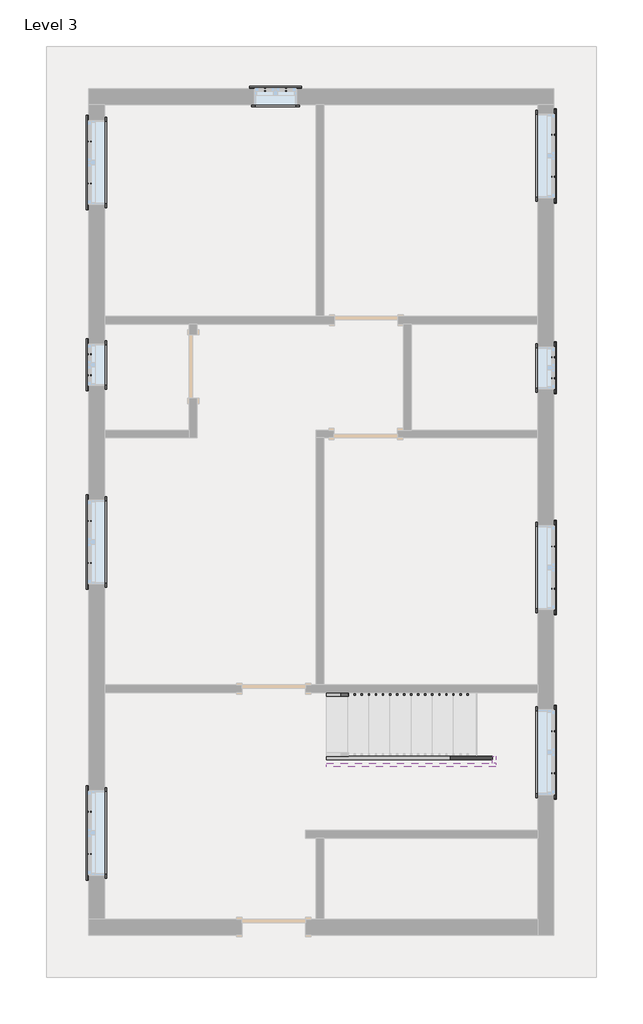
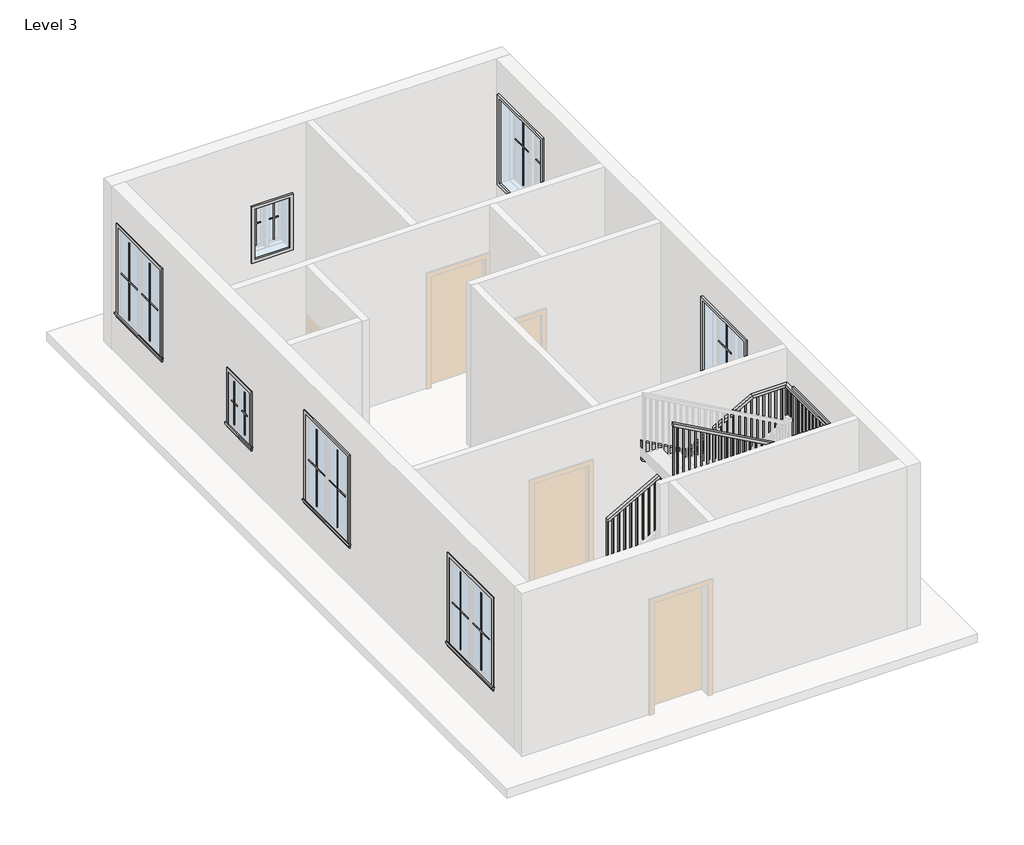
# One storey, part 2 of 2: 36 proxies, 3 members, 1 railing.
"""IFC4 building model written with IfcOpenShell, lengths in millimetres."""

from ifc_helpers import new_model, si_unit, frame, origin, place, context, project, spatial, polyline, outline, extrude, faceted_brep, transform, mapped, element, save
from components import muntin_pattern_2x2_muntin_pattern_2x2_6dad3731, muntin_pattern_2x2_muntin_pattern_2x2_a30a3345, muntin_pattern_2x2_muntin_pattern_2x2_53152e2c, muntin_pattern_2x2_muntin_pattern_2x2_e8f3e573, trim_window_exterior_flat_with_sill_92b9b949, trim_window_exterior_flat_with_sill_a665a915, trim_window_interior_flat_picture_frame_3bb882cf, trim_window_interior_flat_picture_frame_d485c387

model = new_model("IFC4")

# Units and contexts
model_context = context("Model", 3, world=origin())
ifc_project = project(units=[si_unit("LENGTHUNIT", "METRE", prefix="MILLI")], contexts=[model_context])

# Site, building, storey
site = spatial("IfcSite", under=ifc_project)
building = spatial("IfcBuilding", under=site)
storey = spatial("IfcBuildingStorey", under=building, Name="Level 3", Elevation=6096.0)

# Proxies
placement = place(None, origin())
muntin_pattern_2x2_muntin_pattern_2x2_shape = muntin_pattern_2x2_muntin_pattern_2x2_6dad3731(model_context)
element("IfcBuildingElementProxy", 1, Name="Muntin Pattern_2x2 : Muntin Pattern_2x2", ObjectType="Muntin Pattern_2x2 : Muntin Pattern_2x2", at=placement, inside=storey, context=model_context, shape_type="MappedRepresentation", body=[
    mapped(muntin_pattern_2x2_muntin_pattern_2x2_shape, transform((1279.525, 2947.4914062, 7080.25), x_axis=(0.0, 1.0, 0.0), y_axis=(-1.0, 0.0, 0.0), z_axis=(0.0, 0.0, 1.0))),
])
element("IfcBuildingElementProxy", 2, Name="Muntin Pattern_2x2 : Muntin Pattern_2x2", ObjectType="Muntin Pattern_2x2 : Muntin Pattern_2x2", at=placement, inside=storey, context=model_context, shape_type="MappedRepresentation", body=[
    mapped(muntin_pattern_2x2_muntin_pattern_2x2_shape, transform((1279.525, 7138.4914062, 7080.25), x_axis=(0.0, 1.0, 0.0), y_axis=(-1.0, 0.0, 0.0), z_axis=(0.0, 0.0, 1.0))),
])
element("IfcBuildingElementProxy", 3, Name="Muntin Pattern_2x2 : Muntin Pattern_2x2", ObjectType="Muntin Pattern_2x2 : Muntin Pattern_2x2", at=placement, inside=storey, context=model_context, shape_type="MappedRepresentation", body=[
    mapped(muntin_pattern_2x2_muntin_pattern_2x2_shape, transform((1279.525, 12605.8414062, 7080.25), x_axis=(0.0, 1.0, 0.0), y_axis=(-1.0, 0.0, 0.0), z_axis=(0.0, 0.0, 1.0))),
])
element("IfcBuildingElementProxy", 4, Name="Muntin Pattern_2x2 : Muntin Pattern_2x2", ObjectType="Muntin Pattern_2x2 : Muntin Pattern_2x2", at=placement, inside=storey, context=model_context, shape_type="MappedRepresentation", body=[
    mapped(muntin_pattern_2x2_muntin_pattern_2x2_shape, transform((7966.075, 13308.0125, 7080.25), x_axis=(0.0, -1.0, 0.0), y_axis=(1.0, 0.0, 0.0), z_axis=(0.0, 0.0, 1.0))),
])
element("IfcBuildingElementProxy", 5, Name="Muntin Pattern_2x2 : Muntin Pattern_2x2", ObjectType="Muntin Pattern_2x2 : Muntin Pattern_2x2", at=placement, inside=storey, context=model_context, shape_type="MappedRepresentation", body=[
    mapped(muntin_pattern_2x2_muntin_pattern_2x2_shape, transform((7966.075, 7377.1125, 7080.25), x_axis=(0.0, -1.0, 0.0), y_axis=(1.0, 0.0, 0.0), z_axis=(0.0, 0.0, 1.0))),
])
element("IfcBuildingElementProxy", 6, Name="Muntin Pattern_2x2 : Muntin Pattern_2x2", ObjectType="Muntin Pattern_2x2 : Muntin Pattern_2x2", at=placement, inside=storey, context=model_context, shape_type="MappedRepresentation", body=[
    mapped(muntin_pattern_2x2_muntin_pattern_2x2_shape, transform((7966.075, 4716.4625, 7080.25), x_axis=(0.0, -1.0, 0.0), y_axis=(1.0, 0.0, 0.0), z_axis=(0.0, 0.0, 1.0))),
])
muntin_pattern_2x2_muntin_pattern_2x2_2_shape = muntin_pattern_2x2_muntin_pattern_2x2_a30a3345(model_context)
element("IfcBuildingElementProxy", 7, Name="Muntin Pattern_2x2 : Muntin Pattern_2x2", ObjectType="Muntin Pattern_2x2 : Muntin Pattern_2x2", at=placement, inside=storey, context=model_context, shape_type="MappedRepresentation", body=[
    mapped(muntin_pattern_2x2_muntin_pattern_2x2_2_shape, transform((1279.525, 3553.9164063, 7080.25), x_axis=(0.0, -1.0, 0.0), y_axis=(1.0, 0.0, 0.0), z_axis=(0.0, 0.0, 1.0))),
])
element("IfcBuildingElementProxy", 8, Name="Muntin Pattern_2x2 : Muntin Pattern_2x2", ObjectType="Muntin Pattern_2x2 : Muntin Pattern_2x2", at=placement, inside=storey, context=model_context, shape_type="MappedRepresentation", body=[
    mapped(muntin_pattern_2x2_muntin_pattern_2x2_2_shape, transform((1279.525, 7744.9164062, 7080.25), x_axis=(0.0, -1.0, 0.0), y_axis=(1.0, 0.0, 0.0), z_axis=(0.0, 0.0, 1.0))),
])
element("IfcBuildingElementProxy", 9, Name="Muntin Pattern_2x2 : Muntin Pattern_2x2", ObjectType="Muntin Pattern_2x2 : Muntin Pattern_2x2", at=placement, inside=storey, context=model_context, shape_type="MappedRepresentation", body=[
    mapped(muntin_pattern_2x2_muntin_pattern_2x2_2_shape, transform((1279.525, 13212.2664062, 7080.25), x_axis=(0.0, -1.0, 0.0), y_axis=(1.0, 0.0, 0.0), z_axis=(0.0, 0.0, 1.0))),
])
element("IfcBuildingElementProxy", 10, Name="Muntin Pattern_2x2 : Muntin Pattern_2x2", ObjectType="Muntin Pattern_2x2 : Muntin Pattern_2x2", at=placement, inside=storey, context=model_context, shape_type="MappedRepresentation", body=[
    mapped(muntin_pattern_2x2_muntin_pattern_2x2_2_shape, transform((7966.075, 12701.5875, 7080.25), x_axis=(0.0, 1.0, 0.0), y_axis=(-1.0, 0.0, 0.0), z_axis=(0.0, 0.0, 1.0))),
])
element("IfcBuildingElementProxy", 11, Name="Muntin Pattern_2x2 : Muntin Pattern_2x2", ObjectType="Muntin Pattern_2x2 : Muntin Pattern_2x2", at=placement, inside=storey, context=model_context, shape_type="MappedRepresentation", body=[
    mapped(muntin_pattern_2x2_muntin_pattern_2x2_2_shape, transform((7966.075, 6770.6875, 7080.25), x_axis=(0.0, 1.0, 0.0), y_axis=(-1.0, 0.0, 0.0), z_axis=(0.0, 0.0, 1.0))),
])
element("IfcBuildingElementProxy", 12, Name="Muntin Pattern_2x2 : Muntin Pattern_2x2", ObjectType="Muntin Pattern_2x2 : Muntin Pattern_2x2", at=placement, inside=storey, context=model_context, shape_type="MappedRepresentation", body=[
    mapped(muntin_pattern_2x2_muntin_pattern_2x2_2_shape, transform((7966.075, 4110.0375, 7080.25), x_axis=(0.0, 1.0, 0.0), y_axis=(-1.0, 0.0, 0.0), z_axis=(0.0, 0.0, 1.0))),
])
muntin_pattern_2x2_muntin_pattern_2x2_3_shape = muntin_pattern_2x2_muntin_pattern_2x2_53152e2c(model_context)
element("IfcBuildingElementProxy", 13, Name="Muntin Pattern_2x2 : Muntin Pattern_2x2", ObjectType="Muntin Pattern_2x2 : Muntin Pattern_2x2", at=placement, inside=storey, context=model_context, shape_type="MappedRepresentation", body=[
    mapped(muntin_pattern_2x2_muntin_pattern_2x2_3_shape, transform((3811.5875, 13960.475, 7080.25), x_axis=(1.0, 0.0, 0.0), y_axis=(0.0, 1.0, 0.0), z_axis=(0.0, 0.0, 1.0))),
])
element("IfcBuildingElementProxy", 14, Name="Muntin Pattern_2x2 : Muntin Pattern_2x2", ObjectType="Muntin Pattern_2x2 : Muntin Pattern_2x2", at=placement, inside=storey, context=model_context, shape_type="MappedRepresentation", body=[
    mapped(muntin_pattern_2x2_muntin_pattern_2x2_3_shape, transform((7966.075, 10101.2625, 7080.25), x_axis=(0.0, -1.0, 0.0), y_axis=(1.0, 0.0, 0.0), z_axis=(0.0, 0.0, 1.0))),
])
element("IfcBuildingElementProxy", 15, Name="Muntin Pattern_2x2 : Muntin Pattern_2x2", ObjectType="Muntin Pattern_2x2 : Muntin Pattern_2x2", at=placement, inside=storey, context=model_context, shape_type="MappedRepresentation", body=[
    mapped(muntin_pattern_2x2_muntin_pattern_2x2_3_shape, transform((1279.525, 9843.5914062, 7080.25), x_axis=(0.0, 1.0, 0.0), y_axis=(-1.0, 0.0, 0.0), z_axis=(0.0, 0.0, 1.0))),
])
muntin_pattern_2x2_muntin_pattern_2x2_4_shape = muntin_pattern_2x2_muntin_pattern_2x2_e8f3e573(model_context)
element("IfcBuildingElementProxy", 16, Name="Muntin Pattern_2x2 : Muntin Pattern_2x2", ObjectType="Muntin Pattern_2x2 : Muntin Pattern_2x2", at=placement, inside=storey, context=model_context, shape_type="MappedRepresentation", body=[
    mapped(muntin_pattern_2x2_muntin_pattern_2x2_4_shape, transform((4113.2125, 13960.475, 7080.25), x_axis=(-1.0, 0.0, 0.0), y_axis=(0.0, -1.0, 0.0), z_axis=(0.0, 0.0, 1.0))),
])
element("IfcBuildingElementProxy", 17, Name="Muntin Pattern_2x2 : Muntin Pattern_2x2", ObjectType="Muntin Pattern_2x2 : Muntin Pattern_2x2", at=placement, inside=storey, context=model_context, shape_type="MappedRepresentation", body=[
    mapped(muntin_pattern_2x2_muntin_pattern_2x2_4_shape, transform((7966.075, 9799.6375, 7080.25), x_axis=(0.0, 1.0, 0.0), y_axis=(-1.0, 0.0, 0.0), z_axis=(0.0, 0.0, 1.0))),
])
element("IfcBuildingElementProxy", 18, Name="Muntin Pattern_2x2 : Muntin Pattern_2x2", ObjectType="Muntin Pattern_2x2 : Muntin Pattern_2x2", at=placement, inside=storey, context=model_context, shape_type="MappedRepresentation", body=[
    mapped(muntin_pattern_2x2_muntin_pattern_2x2_4_shape, transform((1279.525, 10145.2164062, 7080.25), x_axis=(0.0, -1.0, 0.0), y_axis=(1.0, 0.0, 0.0), z_axis=(0.0, 0.0, 1.0))),
])
trim_window_exterior_flat_with_sill_shape = trim_window_exterior_flat_with_sill_92b9b949(model_context)
element("IfcBuildingElementProxy", 19, Name="Trim-Window-Exterior-Flat : with Sill", ObjectType="Trim-Window-Exterior-Flat : with Sill", at=placement, inside=storey, context=model_context, shape_type="MappedRepresentation", body=[
    mapped(trim_window_exterior_flat_with_sill_shape, transform((1270.0, 3250.7039063, 8534.4), x_axis=(0.0, -1.0, 0.0), y_axis=(0.0, 0.0, 1.0), z_axis=(-1.0, 0.0, 0.0))),
])
element("IfcBuildingElementProxy", 20, Name="Trim-Window-Exterior-Flat : with Sill", ObjectType="Trim-Window-Exterior-Flat : with Sill", at=placement, inside=storey, context=model_context, shape_type="MappedRepresentation", body=[
    mapped(trim_window_exterior_flat_with_sill_shape, transform((1270.0, 7441.7039063, 8534.4), x_axis=(0.0, -1.0, 0.0), y_axis=(0.0, 0.0, 1.0), z_axis=(-1.0, 0.0, 0.0))),
])
element("IfcBuildingElementProxy", 21, Name="Trim-Window-Exterior-Flat : with Sill", ObjectType="Trim-Window-Exterior-Flat : with Sill", at=placement, inside=storey, context=model_context, shape_type="MappedRepresentation", body=[
    mapped(trim_window_exterior_flat_with_sill_shape, transform((1270.0, 12909.0539063, 8534.4), x_axis=(0.0, -1.0, 0.0), y_axis=(0.0, 0.0, 1.0), z_axis=(-1.0, 0.0, 0.0))),
])
element("IfcBuildingElementProxy", 22, Name="Trim-Window-Exterior-Flat : with Sill", ObjectType="Trim-Window-Exterior-Flat : with Sill", at=placement, inside=storey, context=model_context, shape_type="MappedRepresentation", body=[
    mapped(trim_window_exterior_flat_with_sill_shape, transform((7975.6, 13004.8, 8534.4), x_axis=(0.0, 1.0, 0.0), y_axis=(0.0, 0.0, 1.0), z_axis=(1.0, 0.0, 0.0))),
])
element("IfcBuildingElementProxy", 23, Name="Trim-Window-Exterior-Flat : with Sill", ObjectType="Trim-Window-Exterior-Flat : with Sill", at=placement, inside=storey, context=model_context, shape_type="MappedRepresentation", body=[
    mapped(trim_window_exterior_flat_with_sill_shape, transform((7975.6, 7073.9, 8534.4), x_axis=(0.0, 1.0, 0.0), y_axis=(0.0, 0.0, 1.0), z_axis=(1.0, 0.0, 0.0))),
])
element("IfcBuildingElementProxy", 24, Name="Trim-Window-Exterior-Flat : with Sill", ObjectType="Trim-Window-Exterior-Flat : with Sill", at=placement, inside=storey, context=model_context, shape_type="MappedRepresentation", body=[
    mapped(trim_window_exterior_flat_with_sill_shape, transform((7975.6, 4413.25, 8534.4), x_axis=(0.0, 1.0, 0.0), y_axis=(0.0, 0.0, 1.0), z_axis=(1.0, 0.0, 0.0))),
])
trim_window_exterior_flat_with_sill_2_shape = trim_window_exterior_flat_with_sill_a665a915(model_context)
element("IfcBuildingElementProxy", 25, Name="Trim-Window-Exterior-Flat : with Sill", ObjectType="Trim-Window-Exterior-Flat : with Sill", at=placement, inside=storey, context=model_context, shape_type="MappedRepresentation", body=[
    mapped(trim_window_exterior_flat_with_sill_2_shape, transform((3962.4, 13970.0, 7924.8), x_axis=(-1.0, 0.0, 0.0), y_axis=(0.0, 0.0, 1.0), z_axis=(0.0, 1.0, 0.0))),
])
element("IfcBuildingElementProxy", 26, Name="Trim-Window-Exterior-Flat : with Sill", ObjectType="Trim-Window-Exterior-Flat : with Sill", at=placement, inside=storey, context=model_context, shape_type="MappedRepresentation", body=[
    mapped(trim_window_exterior_flat_with_sill_2_shape, transform((7975.6, 9950.45, 7924.8), x_axis=(0.0, 1.0, 0.0), y_axis=(0.0, 0.0, 1.0), z_axis=(1.0, 0.0, 0.0))),
])
element("IfcBuildingElementProxy", 27, Name="Trim-Window-Exterior-Flat : with Sill", ObjectType="Trim-Window-Exterior-Flat : with Sill", at=placement, inside=storey, context=model_context, shape_type="MappedRepresentation", body=[
    mapped(trim_window_exterior_flat_with_sill_2_shape, transform((1270.0, 9994.4039062, 7924.8), x_axis=(0.0, -1.0, 0.0), y_axis=(0.0, 0.0, 1.0), z_axis=(-1.0, 0.0, 0.0))),
])
trim_window_interior_flat_picture_frame_shape = trim_window_interior_flat_picture_frame_3bb882cf(model_context)
element("IfcBuildingElementProxy", 28, Name="Trim-Window-Interior-Flat : Picture Frame", ObjectType="Trim-Window-Interior-Flat : Picture Frame", at=placement, inside=storey, context=model_context, shape_type="MappedRepresentation", body=[
    mapped(trim_window_interior_flat_picture_frame_shape, transform((1498.6, 3250.7039063, 8534.4), x_axis=(0.0, 1.0, 0.0), y_axis=(0.0, 0.0, 1.0), z_axis=(1.0, 0.0, 0.0))),
])
element("IfcBuildingElementProxy", 29, Name="Trim-Window-Interior-Flat : Picture Frame", ObjectType="Trim-Window-Interior-Flat : Picture Frame", at=placement, inside=storey, context=model_context, shape_type="MappedRepresentation", body=[
    mapped(trim_window_interior_flat_picture_frame_shape, transform((1498.6, 7441.7039062, 8534.4), x_axis=(0.0, 1.0, 0.0), y_axis=(0.0, 0.0, 1.0), z_axis=(1.0, 0.0, 0.0))),
])
element("IfcBuildingElementProxy", 30, Name="Trim-Window-Interior-Flat : Picture Frame", ObjectType="Trim-Window-Interior-Flat : Picture Frame", at=placement, inside=storey, context=model_context, shape_type="MappedRepresentation", body=[
    mapped(trim_window_interior_flat_picture_frame_shape, transform((1498.6, 12909.0539062, 8534.4), x_axis=(0.0, 1.0, 0.0), y_axis=(0.0, 0.0, 1.0), z_axis=(1.0, 0.0, 0.0))),
])
element("IfcBuildingElementProxy", 31, Name="Trim-Window-Interior-Flat : Picture Frame", ObjectType="Trim-Window-Interior-Flat : Picture Frame", at=placement, inside=storey, context=model_context, shape_type="MappedRepresentation", body=[
    mapped(trim_window_interior_flat_picture_frame_shape, transform((7747.0, 13004.8, 8534.4), x_axis=(0.0, -1.0, 0.0), y_axis=(0.0, 0.0, 1.0), z_axis=(-1.0, 0.0, 0.0))),
])
element("IfcBuildingElementProxy", 32, Name="Trim-Window-Interior-Flat : Picture Frame", ObjectType="Trim-Window-Interior-Flat : Picture Frame", at=placement, inside=storey, context=model_context, shape_type="MappedRepresentation", body=[
    mapped(trim_window_interior_flat_picture_frame_shape, transform((7747.0, 7073.9, 8534.4), x_axis=(0.0, -1.0, 0.0), y_axis=(0.0, 0.0, 1.0), z_axis=(-1.0, 0.0, 0.0))),
])
element("IfcBuildingElementProxy", 33, Name="Trim-Window-Interior-Flat : Picture Frame", ObjectType="Trim-Window-Interior-Flat : Picture Frame", at=placement, inside=storey, context=model_context, shape_type="MappedRepresentation", body=[
    mapped(trim_window_interior_flat_picture_frame_shape, transform((7747.0, 4413.25, 8534.4), x_axis=(0.0, -1.0, 0.0), y_axis=(0.0, 0.0, 1.0), z_axis=(-1.0, 0.0, 0.0))),
])
trim_window_interior_flat_picture_frame_2_shape = trim_window_interior_flat_picture_frame_d485c387(model_context)
element("IfcBuildingElementProxy", 34, Name="Trim-Window-Interior-Flat : Picture Frame", ObjectType="Trim-Window-Interior-Flat : Picture Frame", at=placement, inside=storey, context=model_context, shape_type="MappedRepresentation", body=[
    mapped(trim_window_interior_flat_picture_frame_2_shape, transform((3962.4, 13741.4, 7924.8), x_axis=(1.0, 0.0, 0.0), y_axis=(0.0, 0.0, 1.0), z_axis=(0.0, -1.0, 0.0))),
])
element("IfcBuildingElementProxy", 35, Name="Trim-Window-Interior-Flat : Picture Frame", ObjectType="Trim-Window-Interior-Flat : Picture Frame", at=placement, inside=storey, context=model_context, shape_type="MappedRepresentation", body=[
    mapped(trim_window_interior_flat_picture_frame_2_shape, transform((7747.0, 9950.45, 7924.8), x_axis=(0.0, -1.0, 0.0), y_axis=(0.0, 0.0, 1.0), z_axis=(-1.0, 0.0, 0.0))),
])
element("IfcBuildingElementProxy", 36, Name="Trim-Window-Interior-Flat : Picture Frame", ObjectType="Trim-Window-Interior-Flat : Picture Frame", at=placement, inside=storey, context=model_context, shape_type="MappedRepresentation", body=[
    mapped(trim_window_interior_flat_picture_frame_2_shape, transform((1498.6, 9994.4039062, 7924.8), x_axis=(0.0, 1.0, 0.0), y_axis=(0.0, 0.0, 1.0), z_axis=(1.0, 0.0, 0.0))),
])

# Members
element("IfcMember", 37, ObjectType="Stringer - 2\" Width", at=placement, inside=storey, context=model_context, shape_type="SweptSolid", body=[
    extrude(outline(polyline([(6303.5983948, 4699.0), (6096.0, 4699.0), (6096.0, 4952.9445028), (7281.3641651, 7086.6), (7630.0428392, 7086.6), (6303.5983948, 4699.0)])), frame((0.0, 4305.3, 0.0), z_axis=(0.0, 1.0, 0.0), x_axis=(0.0, 0.0, 1.0)), (0.0, 0.0, 1.0), 50.8),
])
element("IfcMember", 38, ObjectType="Stringer - 2\" Width", at=placement, inside=storey, context=model_context, shape_type="SweptSolid", body=[
    extrude(outline(polyline([(7086.6, 4356.1), (7137.4, 4356.1), (7137.4, 4254.5), (7086.6, 4254.5), (7086.6, 4356.1)])), frame((0.0, 0.0, 7391.4), z_axis=(0.0, 0.0, 1.0), x_axis=(1.0, 0.0, 0.0)), (0.0, 0.0, 1.0), 304.8),
])
element("IfcMember", 39, ObjectType="Stringer - 2\" Width", at=placement, inside=storey, context=model_context, shape_type="SweptSolid", body=[
    extrude(outline(polyline([(7478.9197207, 7137.4), (7827.5983948, 7137.4), (9182.2650614, 4699.0), (8833.5863873, 4699.0), (7478.9197207, 7137.4)])), frame((0.0, 4203.7, 0.0), z_axis=(0.0, 1.0, 0.0), x_axis=(0.0, 0.0, 1.0)), (0.0, 0.0, 1.0), 50.8),
])

# Railing
element("IfcRailing", 40, ObjectType="Handrail - Rectangular", at=placement, inside=storey, context=model_context, shape_type="SolidModel", body=[
    faceted_brep([(4699.0, 5270.5, 7179.7333333), (4699.0, 5270.5, 7121.620221), (4699.0, 5219.7, 7121.620221), (4699.0, 5219.7, 7179.7333333), (7137.4, 5270.5, 8534.4), (7150.5636022, 5270.5, 8483.6), (7150.5636022, 5219.7, 8483.6), (7137.4, 5219.7, 8534.4), (7747.0, 5270.5, 8534.4), (7747.0, 5270.5, 8483.6), (7696.2, 5219.7, 8483.6), (7696.2, 5219.7, 8534.4), (7747.0, 3289.3, 8534.4), (7747.0, 3289.3, 8483.6), (7696.2, 3340.1, 8483.6), (7696.2, 3340.1, 8534.4), (7442.2, 3289.3, 8534.4), (7429.0363978, 3289.3, 8483.6), (7429.0363978, 3340.1, 8483.6), (7442.2, 3340.1, 8534.4), (4699.0, 3289.3, 10058.4), (4699.0, 3340.1, 10058.4), (4699.0, 3340.1, 10000.2868876), (4699.0, 3289.3, 10000.2868876)], [[[0, 1, 2, 3]], [[1, 0, 4, 5]], [[2, 1, 5, 6]], [[3, 2, 6, 7]], [[0, 3, 7, 4]], [[5, 4, 8, 9]], [[6, 5, 9, 10]], [[7, 6, 10, 11]], [[4, 7, 11, 8]], [[9, 8, 12, 13]], [[10, 9, 13, 14]], [[11, 10, 14, 15]], [[8, 11, 15, 12]], [[13, 12, 16, 17]], [[14, 13, 17, 18]], [[15, 14, 18, 19]], [[12, 15, 19, 16]], [[20, 21, 22, 23]], [[17, 16, 20, 23]], [[18, 17, 23, 22]], [[19, 18, 22, 21]], [[16, 19, 21, 20]]]),
    extrude(outline(polyline([(9963.245221, 4765.675), (8974.6666667, 4765.675), (8974.6666667, 4784.725), (9952.6618876, 4784.725), (9963.245221, 4765.675)])), frame((0.0, 3305.175, 0.0), z_axis=(0.0, 1.0, 0.0), x_axis=(0.0, 0.0, 1.0)), (0.0, 0.0, 1.0), 19.05),
    extrude(outline(polyline([(9906.8007765, 4867.275), (8974.6666667, 4867.275), (8974.6666667, 4886.325), (9896.2174432, 4886.325), (9906.8007765, 4867.275)])), frame((0.0, 3305.175, 0.0), z_axis=(0.0, 1.0, 0.0), x_axis=(0.0, 0.0, 1.0)), (0.0, 0.0, 1.0), 19.05),
    extrude(outline(polyline([(9850.3563321, 4968.875), (8974.6666667, 4968.875), (8974.6666667, 4987.925), (9839.7729988, 4987.925), (9850.3563321, 4968.875)])), frame((0.0, 3305.175, 0.0), z_axis=(0.0, 1.0, 0.0), x_axis=(0.0, 0.0, 1.0)), (0.0, 0.0, 1.0), 19.05),
    extrude(outline(polyline([(9793.9118876, 5070.475), (8805.3333333, 5070.475), (8805.3333333, 5089.525), (9783.3285543, 5089.525), (9793.9118876, 5070.475)])), frame((0.0, 3305.175, 0.0), z_axis=(0.0, 1.0, 0.0), x_axis=(0.0, 0.0, 1.0)), (0.0, 0.0, 1.0), 19.05),
    extrude(outline(polyline([(9737.4674432, 5172.075), (8805.3333333, 5172.075), (8805.3333333, 5191.125), (9726.8841099, 5191.125), (9737.4674432, 5172.075)])), frame((0.0, 3305.175, 0.0), z_axis=(0.0, 1.0, 0.0), x_axis=(0.0, 0.0, 1.0)), (0.0, 0.0, 1.0), 19.05),
    extrude(outline(polyline([(9681.0229988, 5273.675), (8805.3333333, 5273.675), (8805.3333333, 5292.725), (9670.4396654, 5292.725), (9681.0229988, 5273.675)])), frame((0.0, 3305.175, 0.0), z_axis=(0.0, 1.0, 0.0), x_axis=(0.0, 0.0, 1.0)), (0.0, 0.0, 1.0), 19.05),
    extrude(outline(polyline([(9624.5785543, 5375.275), (8636.0, 5375.275), (8636.0, 5394.325), (9613.995221, 5394.325), (9624.5785543, 5375.275)])), frame((0.0, 3305.175, 0.0), z_axis=(0.0, 1.0, 0.0), x_axis=(0.0, 0.0, 1.0)), (0.0, 0.0, 1.0), 19.05),
    extrude(outline(polyline([(9568.1341099, 5476.875), (8636.0, 5476.875), (8636.0, 5495.925), (9557.5507765, 5495.925), (9568.1341099, 5476.875)])), frame((0.0, 3305.175, 0.0), z_axis=(0.0, 1.0, 0.0), x_axis=(0.0, 0.0, 1.0)), (0.0, 0.0, 1.0), 19.05),
    extrude(outline(polyline([(9511.6896654, 5578.475), (8636.0, 5578.475), (8636.0, 5597.525), (9501.1063321, 5597.525), (9511.6896654, 5578.475)])), frame((0.0, 3305.175, 0.0), z_axis=(0.0, 1.0, 0.0), x_axis=(0.0, 0.0, 1.0)), (0.0, 0.0, 1.0), 19.05),
    extrude(outline(polyline([(9455.245221, 5680.075), (8466.6666667, 5680.075), (8466.6666667, 5699.125), (9444.6618876, 5699.125), (9455.245221, 5680.075)])), frame((0.0, 3305.175, 0.0), z_axis=(0.0, 1.0, 0.0), x_axis=(0.0, 0.0, 1.0)), (0.0, 0.0, 1.0), 19.05),
    extrude(outline(polyline([(9398.8007765, 5781.675), (8466.6666667, 5781.675), (8466.6666667, 5800.725), (9388.2174432, 5800.725), (9398.8007765, 5781.675)])), frame((0.0, 3305.175, 0.0), z_axis=(0.0, 1.0, 0.0), x_axis=(0.0, 0.0, 1.0)), (0.0, 0.0, 1.0), 19.05),
    extrude(outline(polyline([(9342.3563321, 5883.275), (8466.6666667, 5883.275), (8466.6666667, 5902.325), (9331.7729988, 5902.325), (9342.3563321, 5883.275)])), frame((0.0, 3305.175, 0.0), z_axis=(0.0, 1.0, 0.0), x_axis=(0.0, 0.0, 1.0)), (0.0, 0.0, 1.0), 19.05),
    extrude(outline(polyline([(9285.9118876, 5984.875), (8297.3333333, 5984.875), (8297.3333333, 6003.925), (9275.3285543, 6003.925), (9285.9118876, 5984.875)])), frame((0.0, 3305.175, 0.0), z_axis=(0.0, 1.0, 0.0), x_axis=(0.0, 0.0, 1.0)), (0.0, 0.0, 1.0), 19.05),
    extrude(outline(polyline([(9229.4674432, 6086.475), (8297.3333333, 6086.475), (8297.3333333, 6105.525), (9218.8841099, 6105.525), (9229.4674432, 6086.475)])), frame((0.0, 3305.175, 0.0), z_axis=(0.0, 1.0, 0.0), x_axis=(0.0, 0.0, 1.0)), (0.0, 0.0, 1.0), 19.05),
    extrude(outline(polyline([(9173.0229988, 6188.075), (8297.3333333, 6188.075), (8297.3333333, 6207.125), (9162.4396654, 6207.125), (9173.0229988, 6188.075)])), frame((0.0, 3305.175, 0.0), z_axis=(0.0, 1.0, 0.0), x_axis=(0.0, 0.0, 1.0)), (0.0, 0.0, 1.0), 19.05),
    extrude(outline(polyline([(9116.5785543, 6289.675), (8128.0, 6289.675), (8128.0, 6308.725), (9105.995221, 6308.725), (9116.5785543, 6289.675)])), frame((0.0, 3305.175, 0.0), z_axis=(0.0, 1.0, 0.0), x_axis=(0.0, 0.0, 1.0)), (0.0, 0.0, 1.0), 19.05),
    extrude(outline(polyline([(9060.1341099, 6391.275), (8128.0, 6391.275), (8128.0, 6410.325), (9049.5507765, 6410.325), (9060.1341099, 6391.275)])), frame((0.0, 3305.175, 0.0), z_axis=(0.0, 1.0, 0.0), x_axis=(0.0, 0.0, 1.0)), (0.0, 0.0, 1.0), 19.05),
    extrude(outline(polyline([(9003.6896654, 6492.875), (8128.0, 6492.875), (8128.0, 6511.925), (8993.1063321, 6511.925), (9003.6896654, 6492.875)])), frame((0.0, 3305.175, 0.0), z_axis=(0.0, 1.0, 0.0), x_axis=(0.0, 0.0, 1.0)), (0.0, 0.0, 1.0), 19.05),
    extrude(outline(polyline([(8947.245221, 6594.475), (7958.6666667, 6594.475), (7958.6666667, 6613.525), (8936.6618876, 6613.525), (8947.245221, 6594.475)])), frame((0.0, 3305.175, 0.0), z_axis=(0.0, 1.0, 0.0), x_axis=(0.0, 0.0, 1.0)), (0.0, 0.0, 1.0), 19.05),
    extrude(outline(polyline([(8890.8007765, 6696.075), (7958.6666667, 6696.075), (7958.6666667, 6715.125), (8880.2174432, 6715.125), (8890.8007765, 6696.075)])), frame((0.0, 3305.175, 0.0), z_axis=(0.0, 1.0, 0.0), x_axis=(0.0, 0.0, 1.0)), (0.0, 0.0, 1.0), 19.05),
    extrude(outline(polyline([(8834.3563321, 6797.675), (7958.6666667, 6797.675), (7958.6666667, 6816.725), (8823.7729988, 6816.725), (8834.3563321, 6797.675)])), frame((0.0, 3305.175, 0.0), z_axis=(0.0, 1.0, 0.0), x_axis=(0.0, 0.0, 1.0)), (0.0, 0.0, 1.0), 19.05),
    extrude(outline(polyline([(8777.9118876, 6899.275), (7789.3333333, 6899.275), (7789.3333333, 6918.325), (8767.3285543, 6918.325), (8777.9118876, 6899.275)])), frame((0.0, 3305.175, 0.0), z_axis=(0.0, 1.0, 0.0), x_axis=(0.0, 0.0, 1.0)), (0.0, 0.0, 1.0), 19.05),
    extrude(outline(polyline([(8721.4674432, 7000.875), (7789.3333333, 7000.875), (7789.3333333, 7019.925), (8710.8841099, 7019.925), (8721.4674432, 7000.875)])), frame((0.0, 3305.175, 0.0), z_axis=(0.0, 1.0, 0.0), x_axis=(0.0, 0.0, 1.0)), (0.0, 0.0, 1.0), 19.05),
    extrude(outline(polyline([(8665.0229988, 7102.475), (7789.3333333, 7102.475), (7789.3333333, 7121.525), (8654.4396654, 7121.525), (8665.0229988, 7102.475)])), frame((0.0, 3305.175, 0.0), z_axis=(0.0, 1.0, 0.0), x_axis=(0.0, 0.0, 1.0)), (0.0, 0.0, 1.0), 19.05),
    extrude(outline(polyline([(8608.5785543, 7204.075), (7620.0, 7204.075), (7620.0, 7223.125), (8597.995221, 7223.125), (8608.5785543, 7204.075)])), frame((0.0, 3305.175, 0.0), z_axis=(0.0, 1.0, 0.0), x_axis=(0.0, 0.0, 1.0)), (0.0, 0.0, 1.0), 19.05),
    extrude(outline(polyline([(8552.1341099, 7305.675), (7620.0, 7305.675), (7620.0, 7324.725), (8541.5507765, 7324.725), (8552.1341099, 7305.675)])), frame((0.0, 3305.175, 0.0), z_axis=(0.0, 1.0, 0.0), x_axis=(0.0, 0.0, 1.0)), (0.0, 0.0, 1.0), 19.05),
    extrude(outline(polyline([(8495.6896654, 7407.275), (7620.0, 7407.275), (7620.0, 7426.325), (8485.1063321, 7426.325), (8495.6896654, 7407.275)])), frame((0.0, 3305.175, 0.0), z_axis=(0.0, 1.0, 0.0), x_axis=(0.0, 0.0, 1.0)), (0.0, 0.0, 1.0), 19.05),
    extrude(outline(polyline([(7527.925, 3305.175), (7508.875, 3305.175), (7508.875, 3324.225), (7527.925, 3324.225), (7527.925, 3305.175)])), frame((0.0, 0.0, 7620.0), z_axis=(0.0, 0.0, 1.0), x_axis=(1.0, 0.0, 0.0)), (0.0, 0.0, 1.0), 863.6),
    extrude(outline(polyline([(7629.525, 3305.175), (7610.475, 3305.175), (7610.475, 3324.225), (7629.525, 3324.225), (7629.525, 3305.175)])), frame((0.0, 0.0, 7620.0), z_axis=(0.0, 0.0, 1.0), x_axis=(1.0, 0.0, 0.0)), (0.0, 0.0, 1.0), 863.6),
    extrude(outline(polyline([(7731.125, 3425.825), (7731.125, 3406.775), (7712.075, 3406.775), (7712.075, 3425.825), (7731.125, 3425.825)])), frame((0.0, 0.0, 7620.0), z_axis=(0.0, 0.0, 1.0), x_axis=(1.0, 0.0, 0.0)), (0.0, 0.0, 1.0), 863.6),
    extrude(outline(polyline([(7731.125, 3527.425), (7731.125, 3508.375), (7712.075, 3508.375), (7712.075, 3527.425), (7731.125, 3527.425)])), frame((0.0, 0.0, 7620.0), z_axis=(0.0, 0.0, 1.0), x_axis=(1.0, 0.0, 0.0)), (0.0, 0.0, 1.0), 863.6),
    extrude(outline(polyline([(7731.125, 3629.025), (7731.125, 3609.975), (7712.075, 3609.975), (7712.075, 3629.025), (7731.125, 3629.025)])), frame((0.0, 0.0, 7620.0), z_axis=(0.0, 0.0, 1.0), x_axis=(1.0, 0.0, 0.0)), (0.0, 0.0, 1.0), 863.6),
    extrude(outline(polyline([(7731.125, 3730.625), (7731.125, 3711.575), (7712.075, 3711.575), (7712.075, 3730.625), (7731.125, 3730.625)])), frame((0.0, 0.0, 7620.0), z_axis=(0.0, 0.0, 1.0), x_axis=(1.0, 0.0, 0.0)), (0.0, 0.0, 1.0), 863.6),
    extrude(outline(polyline([(7731.125, 3832.225), (7731.125, 3813.175), (7712.075, 3813.175), (7712.075, 3832.225), (7731.125, 3832.225)])), frame((0.0, 0.0, 7620.0), z_axis=(0.0, 0.0, 1.0), x_axis=(1.0, 0.0, 0.0)), (0.0, 0.0, 1.0), 863.6),
    extrude(outline(polyline([(7731.125, 3933.825), (7731.125, 3914.775), (7712.075, 3914.775), (7712.075, 3933.825), (7731.125, 3933.825)])), frame((0.0, 0.0, 7620.0), z_axis=(0.0, 0.0, 1.0), x_axis=(1.0, 0.0, 0.0)), (0.0, 0.0, 1.0), 863.6),
    extrude(outline(polyline([(7731.125, 4035.425), (7731.125, 4016.375), (7712.075, 4016.375), (7712.075, 4035.425), (7731.125, 4035.425)])), frame((0.0, 0.0, 7620.0), z_axis=(0.0, 0.0, 1.0), x_axis=(1.0, 0.0, 0.0)), (0.0, 0.0, 1.0), 863.6),
    extrude(outline(polyline([(7731.125, 4137.025), (7731.125, 4117.975), (7712.075, 4117.975), (7712.075, 4137.025), (7731.125, 4137.025)])), frame((0.0, 0.0, 7620.0), z_axis=(0.0, 0.0, 1.0), x_axis=(1.0, 0.0, 0.0)), (0.0, 0.0, 1.0), 863.6),
    extrude(outline(polyline([(7731.125, 4238.625), (7731.125, 4219.575), (7712.075, 4219.575), (7712.075, 4238.625), (7731.125, 4238.625)])), frame((0.0, 0.0, 7620.0), z_axis=(0.0, 0.0, 1.0), x_axis=(1.0, 0.0, 0.0)), (0.0, 0.0, 1.0), 863.6),
    extrude(outline(polyline([(7731.125, 4340.225), (7731.125, 4321.175), (7712.075, 4321.175), (7712.075, 4340.225), (7731.125, 4340.225)])), frame((0.0, 0.0, 7620.0), z_axis=(0.0, 0.0, 1.0), x_axis=(1.0, 0.0, 0.0)), (0.0, 0.0, 1.0), 863.6),
    extrude(outline(polyline([(7731.125, 4441.825), (7731.125, 4422.775), (7712.075, 4422.775), (7712.075, 4441.825), (7731.125, 4441.825)])), frame((0.0, 0.0, 7620.0), z_axis=(0.0, 0.0, 1.0), x_axis=(1.0, 0.0, 0.0)), (0.0, 0.0, 1.0), 863.6),
    extrude(outline(polyline([(7731.125, 4543.425), (7731.125, 4524.375), (7712.075, 4524.375), (7712.075, 4543.425), (7731.125, 4543.425)])), frame((0.0, 0.0, 7620.0), z_axis=(0.0, 0.0, 1.0), x_axis=(1.0, 0.0, 0.0)), (0.0, 0.0, 1.0), 863.6),
    extrude(outline(polyline([(7731.125, 4645.025), (7731.125, 4625.975), (7712.075, 4625.975), (7712.075, 4645.025), (7731.125, 4645.025)])), frame((0.0, 0.0, 7620.0), z_axis=(0.0, 0.0, 1.0), x_axis=(1.0, 0.0, 0.0)), (0.0, 0.0, 1.0), 863.6),
    extrude(outline(polyline([(7731.125, 4746.625), (7731.125, 4727.575), (7712.075, 4727.575), (7712.075, 4746.625), (7731.125, 4746.625)])), frame((0.0, 0.0, 7620.0), z_axis=(0.0, 0.0, 1.0), x_axis=(1.0, 0.0, 0.0)), (0.0, 0.0, 1.0), 863.6),
    extrude(outline(polyline([(7731.125, 4848.225), (7731.125, 4829.175), (7712.075, 4829.175), (7712.075, 4848.225), (7731.125, 4848.225)])), frame((0.0, 0.0, 7620.0), z_axis=(0.0, 0.0, 1.0), x_axis=(1.0, 0.0, 0.0)), (0.0, 0.0, 1.0), 863.6),
    extrude(outline(polyline([(7731.125, 4949.825), (7731.125, 4930.775), (7712.075, 4930.775), (7712.075, 4949.825), (7731.125, 4949.825)])), frame((0.0, 0.0, 7620.0), z_axis=(0.0, 0.0, 1.0), x_axis=(1.0, 0.0, 0.0)), (0.0, 0.0, 1.0), 863.6),
    extrude(outline(polyline([(7731.125, 5051.425), (7731.125, 5032.375), (7712.075, 5032.375), (7712.075, 5051.425), (7731.125, 5051.425)])), frame((0.0, 0.0, 7620.0), z_axis=(0.0, 0.0, 1.0), x_axis=(1.0, 0.0, 0.0)), (0.0, 0.0, 1.0), 863.6),
    extrude(outline(polyline([(7731.125, 5153.025), (7731.125, 5133.975), (7712.075, 5133.975), (7712.075, 5153.025), (7731.125, 5153.025)])), frame((0.0, 0.0, 7620.0), z_axis=(0.0, 0.0, 1.0), x_axis=(1.0, 0.0, 0.0)), (0.0, 0.0, 1.0), 863.6),
    extrude(outline(polyline([(7635.875, 5254.625), (7654.925, 5254.625), (7654.925, 5235.575), (7635.875, 5235.575), (7635.875, 5254.625)])), frame((0.0, 0.0, 7620.0), z_axis=(0.0, 0.0, 1.0), x_axis=(1.0, 0.0, 0.0)), (0.0, 0.0, 1.0), 863.6),
    extrude(outline(polyline([(7534.275, 5254.625), (7553.325, 5254.625), (7553.325, 5235.575), (7534.275, 5235.575), (7534.275, 5254.625)])), frame((0.0, 0.0, 7620.0), z_axis=(0.0, 0.0, 1.0), x_axis=(1.0, 0.0, 0.0)), (0.0, 0.0, 1.0), 863.6),
    extrude(outline(polyline([(7432.675, 5254.625), (7451.725, 5254.625), (7451.725, 5235.575), (7432.675, 5235.575), (7432.675, 5254.625)])), frame((0.0, 0.0, 7620.0), z_axis=(0.0, 0.0, 1.0), x_axis=(1.0, 0.0, 0.0)), (0.0, 0.0, 1.0), 863.6),
    extrude(outline(polyline([(7331.075, 5254.625), (7350.125, 5254.625), (7350.125, 5235.575), (7331.075, 5235.575), (7331.075, 5254.625)])), frame((0.0, 0.0, 7620.0), z_axis=(0.0, 0.0, 1.0), x_axis=(1.0, 0.0, 0.0)), (0.0, 0.0, 1.0), 863.6),
    extrude(outline(polyline([(7229.475, 5254.625), (7248.525, 5254.625), (7248.525, 5235.575), (7229.475, 5235.575), (7229.475, 5254.625)])), frame((0.0, 0.0, 7620.0), z_axis=(0.0, 0.0, 1.0), x_axis=(1.0, 0.0, 0.0)), (0.0, 0.0, 1.0), 863.6),
    extrude(outline(polyline([(8470.995221, 7127.875), (7620.0, 7127.875), (7620.0, 7146.925), (8481.5785543, 7146.925), (8470.995221, 7127.875)])), frame((0.0, 5235.575, 0.0), z_axis=(0.0, 1.0, 0.0), x_axis=(0.0, 0.0, 1.0)), (0.0, 0.0, 1.0), 19.05),
    extrude(outline(polyline([(8414.5507765, 7026.275), (7450.6666667, 7026.275), (7450.6666667, 7045.325), (8425.1341099, 7045.325), (8414.5507765, 7026.275)])), frame((0.0, 5235.575, 0.0), z_axis=(0.0, 1.0, 0.0), x_axis=(0.0, 0.0, 1.0)), (0.0, 0.0, 1.0), 19.05),
    extrude(outline(polyline([(8358.1063321, 6924.675), (7450.6666667, 6924.675), (7450.6666667, 6943.725), (8368.6896654, 6943.725), (8358.1063321, 6924.675)])), frame((0.0, 5235.575, 0.0), z_axis=(0.0, 1.0, 0.0), x_axis=(0.0, 0.0, 1.0)), (0.0, 0.0, 1.0), 19.05),
    extrude(outline(polyline([(8301.6618876, 6823.075), (7450.6666667, 6823.075), (7450.6666667, 6842.125), (8312.245221, 6842.125), (8301.6618876, 6823.075)])), frame((0.0, 5235.575, 0.0), z_axis=(0.0, 1.0, 0.0), x_axis=(0.0, 0.0, 1.0)), (0.0, 0.0, 1.0), 19.05),
    extrude(outline(polyline([(8245.2174432, 6721.475), (7281.3333333, 6721.475), (7281.3333333, 6740.525), (8255.8007765, 6740.525), (8245.2174432, 6721.475)])), frame((0.0, 5235.575, 0.0), z_axis=(0.0, 1.0, 0.0), x_axis=(0.0, 0.0, 1.0)), (0.0, 0.0, 1.0), 19.05),
    extrude(outline(polyline([(8188.7729988, 6619.875), (7281.3333333, 6619.875), (7281.3333333, 6638.925), (8199.3563321, 6638.925), (8188.7729988, 6619.875)])), frame((0.0, 5235.575, 0.0), z_axis=(0.0, 1.0, 0.0), x_axis=(0.0, 0.0, 1.0)), (0.0, 0.0, 1.0), 19.05),
    extrude(outline(polyline([(8132.3285543, 6518.275), (7281.3333333, 6518.275), (7281.3333333, 6537.325), (8142.9118876, 6537.325), (8132.3285543, 6518.275)])), frame((0.0, 5235.575, 0.0), z_axis=(0.0, 1.0, 0.0), x_axis=(0.0, 0.0, 1.0)), (0.0, 0.0, 1.0), 19.05),
    extrude(outline(polyline([(8075.8841099, 6416.675), (7112.0, 6416.675), (7112.0, 6435.725), (8086.4674432, 6435.725), (8075.8841099, 6416.675)])), frame((0.0, 5235.575, 0.0), z_axis=(0.0, 1.0, 0.0), x_axis=(0.0, 0.0, 1.0)), (0.0, 0.0, 1.0), 19.05),
    extrude(outline(polyline([(8019.4396654, 6315.075), (7112.0, 6315.075), (7112.0, 6334.125), (8030.0229988, 6334.125), (8019.4396654, 6315.075)])), frame((0.0, 5235.575, 0.0), z_axis=(0.0, 1.0, 0.0), x_axis=(0.0, 0.0, 1.0)), (0.0, 0.0, 1.0), 19.05),
    extrude(outline(polyline([(7962.995221, 6213.475), (7112.0, 6213.475), (7112.0, 6232.525), (7973.5785543, 6232.525), (7962.995221, 6213.475)])), frame((0.0, 5235.575, 0.0), z_axis=(0.0, 1.0, 0.0), x_axis=(0.0, 0.0, 1.0)), (0.0, 0.0, 1.0), 19.05),
    extrude(outline(polyline([(7906.5507765, 6111.875), (6942.6666667, 6111.875), (6942.6666667, 6130.925), (7917.1341099, 6130.925), (7906.5507765, 6111.875)])), frame((0.0, 5235.575, 0.0), z_axis=(0.0, 1.0, 0.0), x_axis=(0.0, 0.0, 1.0)), (0.0, 0.0, 1.0), 19.05),
    extrude(outline(polyline([(7850.1063321, 6010.275), (6942.6666667, 6010.275), (6942.6666667, 6029.325), (7860.6896654, 6029.325), (7850.1063321, 6010.275)])), frame((0.0, 5235.575, 0.0), z_axis=(0.0, 1.0, 0.0), x_axis=(0.0, 0.0, 1.0)), (0.0, 0.0, 1.0), 19.05),
    extrude(outline(polyline([(7793.6618876, 5908.675), (6942.6666667, 5908.675), (6942.6666667, 5927.725), (7804.245221, 5927.725), (7793.6618876, 5908.675)])), frame((0.0, 5235.575, 0.0), z_axis=(0.0, 1.0, 0.0), x_axis=(0.0, 0.0, 1.0)), (0.0, 0.0, 1.0), 19.05),
    extrude(outline(polyline([(7737.2174432, 5807.075), (6773.3333333, 5807.075), (6773.3333333, 5826.125), (7747.8007765, 5826.125), (7737.2174432, 5807.075)])), frame((0.0, 5235.575, 0.0), z_axis=(0.0, 1.0, 0.0), x_axis=(0.0, 0.0, 1.0)), (0.0, 0.0, 1.0), 19.05),
    extrude(outline(polyline([(7680.7729988, 5705.475), (6773.3333333, 5705.475), (6773.3333333, 5724.525), (7691.3563321, 5724.525), (7680.7729988, 5705.475)])), frame((0.0, 5235.575, 0.0), z_axis=(0.0, 1.0, 0.0), x_axis=(0.0, 0.0, 1.0)), (0.0, 0.0, 1.0), 19.05),
    extrude(outline(polyline([(7624.3285543, 5603.875), (6773.3333333, 5603.875), (6773.3333333, 5622.925), (7634.9118876, 5622.925), (7624.3285543, 5603.875)])), frame((0.0, 5235.575, 0.0), z_axis=(0.0, 1.0, 0.0), x_axis=(0.0, 0.0, 1.0)), (0.0, 0.0, 1.0), 19.05),
    extrude(outline(polyline([(7567.8841099, 5502.275), (6604.0, 5502.275), (6604.0, 5521.325), (7578.4674432, 5521.325), (7567.8841099, 5502.275)])), frame((0.0, 5235.575, 0.0), z_axis=(0.0, 1.0, 0.0), x_axis=(0.0, 0.0, 1.0)), (0.0, 0.0, 1.0), 19.05),
    extrude(outline(polyline([(7511.4396654, 5400.675), (6604.0, 5400.675), (6604.0, 5419.725), (7522.0229988, 5419.725), (7511.4396654, 5400.675)])), frame((0.0, 5235.575, 0.0), z_axis=(0.0, 1.0, 0.0), x_axis=(0.0, 0.0, 1.0)), (0.0, 0.0, 1.0), 19.05),
    extrude(outline(polyline([(7454.995221, 5299.075), (6604.0, 5299.075), (6604.0, 5318.125), (7465.5785543, 5318.125), (7454.995221, 5299.075)])), frame((0.0, 5235.575, 0.0), z_axis=(0.0, 1.0, 0.0), x_axis=(0.0, 0.0, 1.0)), (0.0, 0.0, 1.0), 19.05),
    extrude(outline(polyline([(7398.5507765, 5197.475), (6434.6666667, 5197.475), (6434.6666667, 5216.525), (7409.1341099, 5216.525), (7398.5507765, 5197.475)])), frame((0.0, 5235.575, 0.0), z_axis=(0.0, 1.0, 0.0), x_axis=(0.0, 0.0, 1.0)), (0.0, 0.0, 1.0), 19.05),
    extrude(outline(polyline([(7342.1063321, 5095.875), (6434.6666667, 5095.875), (6434.6666667, 5114.925), (7352.6896654, 5114.925), (7342.1063321, 5095.875)])), frame((0.0, 5235.575, 0.0), z_axis=(0.0, 1.0, 0.0), x_axis=(0.0, 0.0, 1.0)), (0.0, 0.0, 1.0), 19.05),
    extrude(outline(polyline([(7285.6618876, 4994.275), (6434.6666667, 4994.275), (6434.6666667, 5013.325), (7296.245221, 5013.325), (7285.6618876, 4994.275)])), frame((0.0, 5235.575, 0.0), z_axis=(0.0, 1.0, 0.0), x_axis=(0.0, 0.0, 1.0)), (0.0, 0.0, 1.0), 19.05),
    extrude(outline(polyline([(7229.2174432, 4892.675), (6265.3333333, 4892.675), (6265.3333333, 4911.725), (7239.8007765, 4911.725), (7229.2174432, 4892.675)])), frame((0.0, 5235.575, 0.0), z_axis=(0.0, 1.0, 0.0), x_axis=(0.0, 0.0, 1.0)), (0.0, 0.0, 1.0), 19.05),
    extrude(outline(polyline([(7172.7729988, 4791.075), (6265.3333333, 4791.075), (6265.3333333, 4810.125), (7183.3563321, 4810.125), (7172.7729988, 4791.075)])), frame((0.0, 5235.575, 0.0), z_axis=(0.0, 1.0, 0.0), x_axis=(0.0, 0.0, 1.0)), (0.0, 0.0, 1.0), 19.05),
    extrude(outline(polyline([(7731.125, 3324.225), (7731.125, 3305.175), (7712.075, 3305.175), (7712.075, 3324.225), (7731.125, 3324.225)])), frame((0.0, 0.0, 7620.0), z_axis=(0.0, 0.0, 1.0), x_axis=(1.0, 0.0, 0.0)), (0.0, 0.0, 1.0), 863.6),
    extrude(outline(polyline([(7712.075, 5254.625), (7731.125, 5254.625), (7731.125, 5235.575), (7712.075, 5235.575), (7712.075, 5254.625)])), frame((0.0, 0.0, 7620.0), z_axis=(0.0, 0.0, 1.0), x_axis=(1.0, 0.0, 0.0)), (0.0, 0.0, 1.0), 863.6),
    extrude(outline(polyline([(10000.2868876, 4699.0), (8974.6666667, 4699.0), (8974.6666667, 4718.05), (9989.7035543, 4718.05), (10000.2868876, 4699.0)])), frame((0.0, 3305.175, 0.0), z_axis=(0.0, 1.0, 0.0), x_axis=(0.0, 0.0, 1.0)), (0.0, 0.0, 1.0), 19.05),
    extrude(outline(polyline([(7121.620221, 4699.0), (6265.3333333, 4699.0), (6265.3333333, 4718.05), (7132.2035543, 4718.05), (7121.620221, 4699.0)])), frame((0.0, 5235.575, 0.0), z_axis=(0.0, 1.0, 0.0), x_axis=(0.0, 0.0, 1.0)), (0.0, 0.0, 1.0), 19.05),
])

save(model, "model.ifc")

# Revit data of these elements
# Type "Muntin Pattern_2x2 : Muntin Pattern_2x2"
#   Width [instance default] = 4' - 0"
#   Thickness = 0' - 0 1/2"
#   Height [instance default] = 4' - 0"
#   Distance = 0' - 0 3/4"
#   Interior Material [instance default] = none
#   Exterior Material [instance default] = none
#   Default Elevation = 0
# Type "Trim-Window-Exterior-Flat : with Sill"
#   Trim Width = 0' - 2 1/4"
#   Trim Thickness_Picture Frame = 0' - 1 1/4"
#   Trim Thickness_with Sill = 0' - 0 3/4"
#   Sill Thickness = 0' - 1 1/4"
#   Opening Width [instance default] = 2' - 0"
#   Opening Height [instance default] = 3' - 0"
#   Default Elevation = 4' - 0"
#   Sill = yes
#   Picture Frame = no
#   Trim Material [instance default] = none
# Type "Trim-Window-Interior-Flat : Picture Frame"
#   Trim Thickness_Picture Frame = 0' - 1 1/4"
#   Trim Width = 0' - 2 1/4"
#   Trim Thickness_with Sill = 0' - 0 3/4"
#   Sill Thickness = 0' - 1 1/4"
#   Opening Width [instance default] = 2' - 0"
#   Opening Height [instance default] = 3' - 0"
#   Default Elevation = 4' - 0"
#   Sill = no
#   Picture Frame = yes
#   Trim Material [instance default] = none
# Type "Handrail - Rectangular"
#   Assembly Code = "C2010400"
#   built-in parameter 1008612 = 0.0416667 (stored number, unit not read)
#   built-in parameter 1008611 = 0.0416667 (stored number, unit not read)
#   built-in parameter 1008609 = 0.333333 (stored number, unit not read)
#   built-in parameter 1008604 = 0.166667 (stored number, unit not read)
#   built-in parameter 1008603 = 0.166667 (stored number, unit not read)
#   Railing Height = 3' - 0"
#   built-in parameter 1008630 = 2
#   built-in parameter 1008610 = 2
#   built-in parameter 1008618 = Baluster - Square : 3/4"
# Elements 1, 2, 3, 4, 5, 6, 7, 8, 9, 10, 11, 12 (IfcBuildingElementProxy, "Muntin Pattern_2x2 : Muntin Pattern_2x2")
#   Width = 1' - 6 5/8"
#   Height = 4' - 6 1/2"
#   Interior Material = Wood - Stained
#   Exterior Material = Clad - White
#   Phase Created = New Construction
#   Materials on its faces: "Clad - White", "Wood - Stained"
# Elements 13, 14, 15, 16, 17, 18 (IfcBuildingElementProxy, "Muntin Pattern_2x2 : Muntin Pattern_2x2")
#   Width = 0' - 6 5/8"
#   Height = 2' - 6 1/2"
#   Interior Material = Wood - Stained
#   Exterior Material = Clad - White
#   Phase Created = New Construction
#   Materials on its faces: "Clad - White", "Wood - Stained"
# Elements 19, 20, 21, 22, 23, 24 (IfcBuildingElementProxy, "Trim-Window-Exterior-Flat : with Sill")
#   Opening Width = 4' - 0"
#   Opening Height = 5' - 0"
#   Trim Material = Clad - White
#   Phase Created = New Construction
#   Materials on its faces: "Clad - White"
# Elements 25, 26, 27 (IfcBuildingElementProxy, "Trim-Window-Exterior-Flat : with Sill")
#   Opening Width = 2' - 0"
#   Opening Height = 3' - 0"
#   Trim Material = Clad - White
#   Phase Created = New Construction
#   Materials on its faces: "Clad - White"
# Elements 28, 29, 30, 31, 32, 33 (IfcBuildingElementProxy, "Trim-Window-Interior-Flat : Picture Frame")
#   Opening Width = 4' - 0"
#   Opening Height = 5' - 0"
#   Trim Material = Wood - Stained
#   Phase Created = New Construction
#   Materials on its faces: "Wood - Stained"
# Elements 34, 35, 36 (IfcBuildingElementProxy, "Trim-Window-Interior-Flat : Picture Frame")
#   Opening Width = 2' - 0"
#   Opening Height = 3' - 0"
#   Trim Material = Wood - Stained
#   Phase Created = New Construction
#   Materials on its faces: "Wood - Stained"
# Elements 37, 38, 39 (IfcMember, "Stringer - 2\" Width")
#   Phase Created = New Construction
# Element 40 (IfcRailing, "Handrail - Rectangular")
#   Phase Created = New Construction
# Materials
#   "Clad - White": class "Wood", colour RGB 242 242 238, transparency 0, Cost = 0
#   "Wood - Stained": class "Wood", colour RGB 224 178 126, transparency 0, Cost = 0
